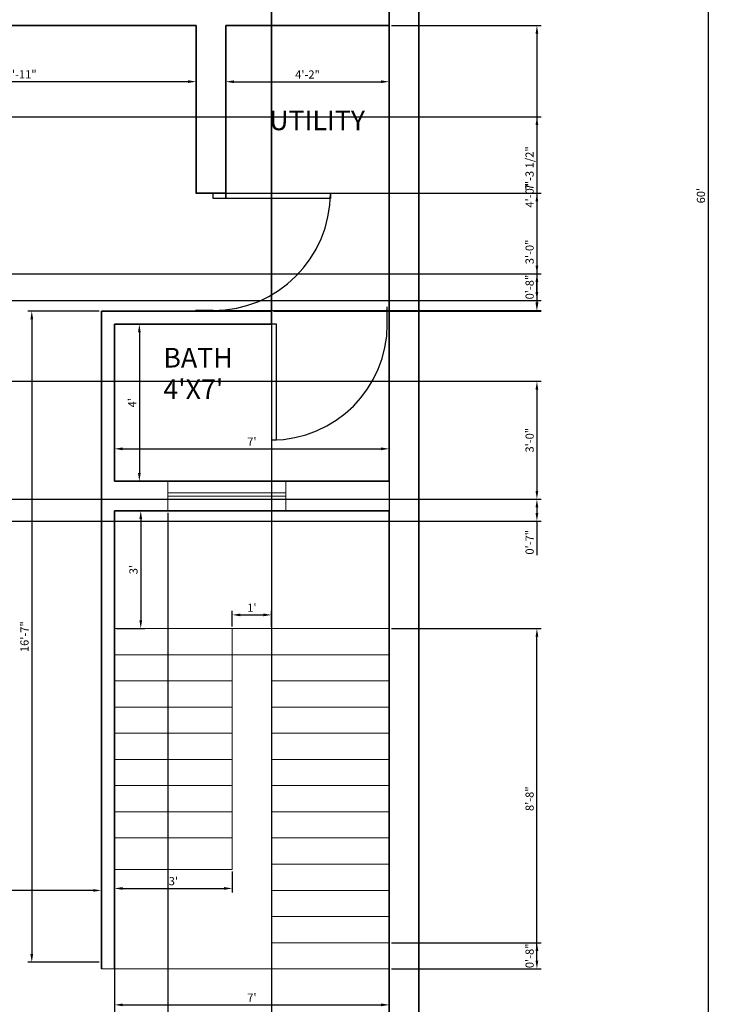
# Model space of a CAD drawing. Units: inches. Extents: x 2178 to 2667, y 1439 to 2239.
# Tile 3 of 5: x 2456 to 2667, y 1590 to 1891. Entities that reach past the tile are written whole.
import ezdxf

# ---------------------------------------------------------------- set-up
doc = ezdxf.new("R2010")
doc.units = ezdxf.units.IN
for name, color, linetype, lineweight in [('A-ANNO-DIMS', 2, 'Continuous', 18), ('A-AREA-IDEN', 7, 'Continuous', 18), ('A-DOOR', 3, 'Continuous', 25), ('A-FLOR-STRS', 7, 'Continuous', 18), ('A-GLAZ', 4, 'Continuous', 18), ('A-WALL', 7, 'Continuous', 35)]:
    doc.layers.add(name, color=color, linetype=linetype, lineweight=lineweight)
doc.styles.get("Standard").update_dxf_attribs({"font": 'arial.ttf'})
doc.dimstyles.new('Copy of ISO-25', dxfattribs={"dimtxt": 2.5, "dimasz": 2.5, "dimexe": 1.25, "dimexo": 0.625, "dimtad": 1, "dimdec": 1, "dimlunit": 4, "dimtxsty": 'Standard', "dimcen": 2.5, "dimadec": 0, "dimazin": 0, "dimtfac": 1, "dimtdec": 1, "dimtmove": 0, "dimatfit": 3, "dimfxl": 1, "dimarcsym": 0})

# ---------------------------------------------------------------- blocks, each defined once
blk = doc.blocks.new('*D14')
at = {"layer": 'A-ANNO-DIMS', "color": 0, "lineweight": -2, "transparency": 16777216}
for p, q in [((2402.53, 1888.41), (2402.53, 1870.62)), ((2509.53, 1888.41), (2509.53, 1870.62)), ((2405.03, 1871.87), (2507.03, 1871.87))]:
    blk.add_line(p, q, dxfattribs=at)
at = {"layer": 'A-ANNO-DIMS', "color": 0, "transparency": 16777216}
for points in [[(2405.03, 1872.29), (2405.03, 1871.45), (2402.53, 1871.87)], [(2507.03, 1872.29), (2507.03, 1871.45), (2509.53, 1871.87)]]:
    blk.add_solid(points, dxfattribs=at)
at = {"layer": 'Defpoints', "color": 0, "transparency": 16777216}
for p in [(2402.53, 1889.03), (2509.53, 1889.03), (2509.53, 1871.87)]:
    blk.add_point(p, dxfattribs=at)
at = {"layer": 'A-ANNO-DIMS', "color": 0, "transparency": 16777216, "insert": (2456.03, 1873.77), "char_height": 2.5, "attachment_point": 5}
blk.add_mtext('8\'-11"', dxfattribs=at)
blk = doc.blocks.new('*U22')
for p, q in [((0, 0), (0, 6)), ((40, 0), (40, 6))]:
    blk.add_line(p, q)
blk.add_lwpolyline([(0, 0), (0, -40), (1.75, -40), (1.75, 0)], close=True)
blk.add_arc((0, 0), 40, 270, 0)
blk = doc.blocks.new('*D29')
at = {"layer": 'A-ANNO-DIMS', "color": 0, "lineweight": -2, "transparency": 16777216}
for p, q in [((2402.53, 1603.39), (2402.53, 1625.96)), ((2478.03, 1624.71), (2405.03, 1624.71)), ((2480.53, 1603.39), (2480.53, 1625.96))]:
    blk.add_line(p, q, dxfattribs=at)
at = {"layer": 'A-ANNO-DIMS', "color": 0, "transparency": 16777216}
for points in [[(2405.03, 1625.13), (2405.03, 1624.3), (2402.53, 1624.71)], [(2478.03, 1625.13), (2478.03, 1624.3), (2480.53, 1624.71)]]:
    blk.add_solid(points, dxfattribs=at)
at = {"layer": 'Defpoints', "color": 0, "transparency": 16777216}
for p in [(2402.53, 1624.71), (2402.53, 1602.76), (2480.53, 1602.76)]:
    blk.add_point(p, dxfattribs=at)
at = {"layer": 'A-ANNO-DIMS', "color": 0, "transparency": 16777216, "insert": (2441.53, 1626.61), "char_height": 2.5, "attachment_point": 5}
blk.add_mtext('6\'-6"', dxfattribs=at)
blk = doc.blocks.new('*D30')
at = {"layer": 'A-ANNO-DIMS', "color": 0, "lineweight": -2, "transparency": 16777216}
for p, q in [((2479.9, 1801.74), (2458.02, 1801.74)), ((2459.27, 1799.24), (2459.27, 1605.26)), ((2479.9, 1602.76), (2458.02, 1602.76))]:
    blk.add_line(p, q, dxfattribs=at)
at = {"layer": 'A-ANNO-DIMS', "color": 0, "transparency": 16777216}
for points in [[(2458.86, 1799.24), (2459.69, 1799.24), (2459.27, 1801.74)], [(2458.86, 1605.26), (2459.69, 1605.26), (2459.27, 1602.76)]]:
    blk.add_solid(points, dxfattribs=at)
at = {"layer": 'Defpoints', "color": 0, "transparency": 16777216}
for p in [(2480.53, 1801.74), (2459.27, 1602.76), (2480.53, 1602.76)]:
    blk.add_point(p, dxfattribs=at)
at = {"layer": 'A-ANNO-DIMS', "color": 0, "transparency": 16777216, "insert": (2457.37, 1702.25), "char_height": 2.5, "attachment_point": 5, "rotation": 90}
blk.add_mtext('16\'-7"', dxfattribs=at)
blk = doc.blocks.new('*D31')
at = {"layer": 'A-ANNO-DIMS', "color": 0, "lineweight": -2, "transparency": 16777216}
for p, q in [((2484.53, 1600.12), (2484.53, 1588.5)), ((2568.53, 1600.12), (2568.53, 1588.5)), ((2487.03, 1589.75), (2566.03, 1589.75))]:
    blk.add_line(p, q, dxfattribs=at)
at = {"layer": 'A-ANNO-DIMS', "color": 0, "transparency": 16777216}
for points in [[(2487.03, 1590.17), (2487.03, 1589.33), (2484.53, 1589.75)], [(2566.03, 1590.17), (2566.03, 1589.33), (2568.53, 1589.75)]]:
    blk.add_solid(points, dxfattribs=at)
at = {"layer": 'Defpoints', "color": 0, "transparency": 16777216}
for p in [(2484.53, 1600.74), (2568.53, 1600.74), (2568.53, 1589.75)]:
    blk.add_point(p, dxfattribs=at)
at = {"layer": 'A-ANNO-DIMS', "color": 0, "transparency": 16777216, "insert": (2526.53, 1591.63), "char_height": 2.5, "attachment_point": 5}
blk.add_mtext("7'", dxfattribs=at)
blk = doc.blocks.new('*D32')
at = {"layer": 'A-ANNO-DIMS', "color": 0, "lineweight": -2, "transparency": 16777216}
for p, q in [((2485.15, 1740.74), (2493.82, 1740.74)), ((2492.57, 1738.24), (2492.57, 1707.24)), ((2485.15, 1704.74), (2493.82, 1704.74))]:
    blk.add_line(p, q, dxfattribs=at)
at = {"layer": 'A-ANNO-DIMS', "color": 0, "transparency": 16777216}
for points in [[(2492.16, 1738.24), (2492.99, 1738.24), (2492.57, 1740.74)], [(2492.16, 1707.24), (2492.99, 1707.24), (2492.57, 1704.74)]]:
    blk.add_solid(points, dxfattribs=at)
at = {"layer": 'Defpoints', "color": 0, "transparency": 16777216}
for p in [(2484.53, 1740.74), (2484.53, 1704.74), (2492.57, 1704.74)]:
    blk.add_point(p, dxfattribs=at)
at = {"layer": 'A-ANNO-DIMS', "color": 0, "transparency": 16777216, "insert": (2490.67, 1722.74), "char_height": 2.5, "attachment_point": 5, "rotation": 90}
blk.add_mtext("3'", dxfattribs=at)
blk = doc.blocks.new('*D33')
at = {"layer": 'A-ANNO-DIMS', "color": 0, "lineweight": -2, "transparency": 16777216}
for p, q in [((2485.15, 1797.74), (2493.39, 1797.74)), ((2492.14, 1795.24), (2492.14, 1752.24)), ((2485.15, 1749.74), (2493.39, 1749.74))]:
    blk.add_line(p, q, dxfattribs=at)
at = {"layer": 'A-ANNO-DIMS', "color": 0, "transparency": 16777216}
for points in [[(2491.73, 1795.24), (2492.56, 1795.24), (2492.14, 1797.74)], [(2491.73, 1752.24), (2492.56, 1752.24), (2492.14, 1749.74)]]:
    blk.add_solid(points, dxfattribs=at)
at = {"layer": 'Defpoints', "color": 0, "transparency": 16777216}
for p in [(2484.53, 1797.74), (2484.53, 1749.74), (2492.14, 1749.74)]:
    blk.add_point(p, dxfattribs=at)
at = {"layer": 'A-ANNO-DIMS', "color": 0, "transparency": 16777216, "insert": (2490.27, 1773.74), "char_height": 2.5, "attachment_point": 5, "rotation": 90}
blk.add_mtext("4'", dxfattribs=at)
blk = doc.blocks.new('*D34')
at = {"layer": 'A-ANNO-DIMS', "color": 0, "lineweight": -2, "transparency": 16777216}
for p, q in [((2484.53, 1750.37), (2484.53, 1760.9)), ((2568.53, 1750.37), (2568.53, 1760.9)), ((2487.03, 1759.65), (2566.03, 1759.65))]:
    blk.add_line(p, q, dxfattribs=at)
at = {"layer": 'A-ANNO-DIMS', "color": 0, "transparency": 16777216}
for points in [[(2487.03, 1760.07), (2487.03, 1759.23), (2484.53, 1759.65)], [(2566.03, 1760.07), (2566.03, 1759.23), (2568.53, 1759.65)]]:
    blk.add_solid(points, dxfattribs=at)
at = {"layer": 'Defpoints', "color": 0, "transparency": 16777216}
for p in [(2568.53, 1759.65), (2484.53, 1749.74), (2568.53, 1749.74)]:
    blk.add_point(p, dxfattribs=at)
at = {"layer": 'A-ANNO-DIMS', "color": 0, "transparency": 16777216, "insert": (2526.53, 1761.52), "char_height": 2.5, "attachment_point": 5}
blk.add_mtext("7'", dxfattribs=at)
blk = doc.blocks.new('*D35')
at = {"layer": 'A-ANNO-DIMS', "color": 0, "lineweight": -2, "transparency": 16777216}
for p, q in [((2518.53, 1888.41), (2518.53, 1870.58)), ((2568.53, 1888.41), (2568.53, 1870.58)), ((2521.03, 1871.83), (2566.03, 1871.83))]:
    blk.add_line(p, q, dxfattribs=at)
at = {"layer": 'A-ANNO-DIMS', "color": 0, "transparency": 16777216}
for points in [[(2521.03, 1872.25), (2521.03, 1871.42), (2518.53, 1871.83)], [(2566.03, 1872.25), (2566.03, 1871.42), (2568.53, 1871.83)]]:
    blk.add_solid(points, dxfattribs=at)
at = {"layer": 'Defpoints', "color": 0, "transparency": 16777216}
for p in [(2518.53, 1889.03), (2568.53, 1889.03), (2568.53, 1871.83)]:
    blk.add_point(p, dxfattribs=at)
at = {"layer": 'A-ANNO-DIMS', "color": 0, "transparency": 16777216, "insert": (2543.53, 1873.71), "char_height": 2.5, "attachment_point": 5}
blk.add_mtext('4\'-2"', dxfattribs=at)
blk = doc.blocks.new('*U23')
for p, q in [((-40, 0), (-40, 6)), ((0, 0), (0, 6))]:
    blk.add_line(p, q)
blk.add_lwpolyline([(0, 0), (0, -40), (-1.75, -40), (-1.75, 0)], close=True)
blk.add_arc((0, 0), 40, 180, 270)
blk = doc.blocks.new('*D38')
at = {"layer": 'A-ANNO-DIMS', "color": 0, "lineweight": -2, "transparency": 16777216}
for p, q in [((2484.53, 1630.51), (2484.53, 1624.07)), ((2520.53, 1630.51), (2520.53, 1624.07)), ((2487.03, 1625.32), (2518.03, 1625.32))]:
    blk.add_line(p, q, dxfattribs=at)
at = {"layer": 'A-ANNO-DIMS', "color": 0, "transparency": 16777216}
for points in [[(2487.03, 1625.74), (2487.03, 1624.91), (2484.53, 1625.32)], [(2518.03, 1625.74), (2518.03, 1624.91), (2520.53, 1625.32)]]:
    blk.add_solid(points, dxfattribs=at)
at = {"layer": 'Defpoints', "color": 0, "transparency": 16777216}
for p in [(2484.53, 1631.13), (2520.53, 1631.13), (2520.53, 1625.32)]:
    blk.add_point(p, dxfattribs=at)
at = {"layer": 'A-ANNO-DIMS', "color": 0, "transparency": 16777216, "insert": (2502.53, 1627.23), "char_height": 2.5, "attachment_point": 5}
blk.add_mtext("3'", dxfattribs=at)
blk = doc.blocks.new('*D39')
at = {"layer": 'A-ANNO-DIMS', "color": 0, "lineweight": -2, "transparency": 16777216}
for p, q in [((2520.53, 1705.37), (2520.53, 1710.16)), ((2532.53, 1705.37), (2532.53, 1710.16)), ((2523.03, 1708.91), (2530.03, 1708.91))]:
    blk.add_line(p, q, dxfattribs=at)
at = {"layer": 'A-ANNO-DIMS', "color": 0, "transparency": 16777216}
for points in [[(2523.03, 1709.33), (2523.03, 1708.49), (2520.53, 1708.91)], [(2530.03, 1709.33), (2530.03, 1708.49), (2532.53, 1708.91)]]:
    blk.add_solid(points, dxfattribs=at)
at = {"layer": 'Defpoints', "color": 0, "transparency": 16777216}
for p in [(2532.53, 1708.91), (2520.53, 1704.74), (2532.53, 1704.74)]:
    blk.add_point(p, dxfattribs=at)
at = {"layer": 'A-ANNO-DIMS', "color": 0, "transparency": 16777216, "insert": (2526.53, 1710.79), "char_height": 2.5, "attachment_point": 5}
blk.add_mtext("1'", dxfattribs=at)
blk = doc.blocks.new('*D41')
at = {"layer": 'A-ANNO-DIMS', "color": 0, "lineweight": -2, "transparency": 16777216}
for p, q in [((2578.15, 2197.03), (2667.22, 2197.03)), ((2665.97, 2194.53), (2665.97, 1479.53)), ((2578.15, 1477.03), (2667.22, 1477.03))]:
    blk.add_line(p, q, dxfattribs=at)
at = {"layer": 'A-ANNO-DIMS', "color": 0, "transparency": 16777216}
for points in [[(2665.56, 2194.53), (2666.39, 2194.53), (2665.97, 2197.03)], [(2665.56, 1479.53), (2666.39, 1479.53), (2665.97, 1477.03)]]:
    blk.add_solid(points, dxfattribs=at)
at = {"layer": 'Defpoints', "color": 0, "transparency": 16777216}
for p in [(2577.53, 2197.03), (2577.53, 1477.03), (2665.97, 1477.03)]:
    blk.add_point(p, dxfattribs=at)
at = {"layer": 'A-ANNO-DIMS', "color": 0, "transparency": 16777216, "insert": (2664.07, 1837.03), "char_height": 2.5, "attachment_point": 5, "rotation": 90}
blk.add_mtext("60'", dxfattribs=at)
blk = doc.blocks.new('WIN-36IN')
for p, q in [((0, 0), (0, 9)), ((36, 9), (36, 0)), ((0, 5.5), (36, 5.5)), ((0, 4.5), (36, 4.5)), ((0, 3.5), (36, 3.5)), ((36, 0), (0, 0))]:
    blk.add_line(p, q)
blk = doc.blocks.new('*D50')
at = {"layer": 'A-ANNO-DIMS', "color": 0, "lineweight": -2, "transparency": 16777216}
for p, q in [((2569.15, 1889.03), (2614.88, 1889.03)), ((2613.63, 1886.53), (2613.63, 1804.24)), ((2533.15, 1801.74), (2614.88, 1801.74))]:
    blk.add_line(p, q, dxfattribs=at)
at = {"layer": 'A-ANNO-DIMS', "color": 0, "transparency": 16777216}
for points in [[(2613.21, 1886.53), (2614.04, 1886.53), (2613.63, 1889.03)], [(2613.21, 1804.24), (2614.04, 1804.24), (2613.63, 1801.74)]]:
    blk.add_solid(points, dxfattribs=at)
at = {"layer": 'Defpoints', "color": 0, "transparency": 16777216}
for p in [(2568.53, 1889.03), (2532.53, 1801.74), (2613.63, 1801.74)]:
    blk.add_point(p, dxfattribs=at)
at = {"layer": 'A-ANNO-DIMS', "color": 0, "transparency": 16777216, "insert": (2611.71, 1845.39), "char_height": 2.5, "attachment_point": 5, "rotation": 90}
blk.add_mtext('7\'-3 1/2"', dxfattribs=at)
blk = doc.blocks.new('*D53')
at = {"layer": 'A-ANNO-DIMS', "color": 0, "lineweight": -2, "transparency": 16777216}
for p, q in [((2274.15, 1861.13), (2614.88, 1861.13)), ((2613.63, 1858.63), (2613.63, 1815.63)), ((2274.15, 1813.13), (2614.88, 1813.13))]:
    blk.add_line(p, q, dxfattribs=at)
at = {"layer": 'A-ANNO-DIMS', "color": 0, "transparency": 16777216}
for points in [[(2613.21, 1858.63), (2614.04, 1858.63), (2613.63, 1861.13)], [(2613.21, 1815.63), (2614.04, 1815.63), (2613.63, 1813.13)]]:
    blk.add_solid(points, dxfattribs=at)
at = {"layer": 'Defpoints', "color": 0, "transparency": 16777216}
for p in [(2273.53, 1861.13), (2273.53, 1813.13), (2613.63, 1813.13)]:
    blk.add_point(p, dxfattribs=at)
at = {"layer": 'A-ANNO-DIMS', "color": 0, "transparency": 16777216, "insert": (2611.72, 1837.13), "char_height": 2.5, "attachment_point": 5, "rotation": 90}
blk.add_mtext('4\'-0"', dxfattribs=at)
blk = doc.blocks.new('*D54')
at = {"layer": 'A-ANNO-DIMS', "color": 0, "lineweight": -2, "transparency": 16777216}
for p, q in [((2274.15, 1813.13), (2614.88, 1813.13)), ((2613.63, 1807.53), (2613.63, 1810.63)), ((2274.15, 1805.03), (2614.88, 1805.03))]:
    blk.add_line(p, q, dxfattribs=at)
at = {"layer": 'A-ANNO-DIMS', "color": 0, "transparency": 16777216}
for points in [[(2613.21, 1810.63), (2614.04, 1810.63), (2613.63, 1813.13)], [(2613.21, 1807.53), (2614.04, 1807.53), (2613.63, 1805.03)]]:
    blk.add_solid(points, dxfattribs=at)
at = {"layer": 'Defpoints', "color": 0, "transparency": 16777216}
for p in [(2273.53, 1813.13), (2613.63, 1813.13), (2273.53, 1805.03)]:
    blk.add_point(p, dxfattribs=at)
at = {"layer": 'A-ANNO-DIMS', "color": 0, "transparency": 16777216, "insert": (2611.72, 1809.08), "char_height": 2.5, "attachment_point": 5, "rotation": 90}
blk.add_mtext('0\'-8"', dxfattribs=at)
blk = doc.blocks.new('*D58')
at = {"layer": 'A-ANNO-DIMS', "color": 0, "lineweight": -2, "transparency": 16777216}
for p, q in [((2484.53, 1740.12), (2484.53, 1439.68)), ((2500.89, 1740.12), (2500.89, 1439.68)), ((2487.03, 1440.93), (2498.39, 1440.93))]:
    blk.add_line(p, q, dxfattribs=at)
at = {"layer": 'A-ANNO-DIMS', "color": 0, "transparency": 16777216}
for points in [[(2487.03, 1441.35), (2487.03, 1440.52), (2484.53, 1440.93)], [(2498.39, 1441.35), (2498.39, 1440.52), (2500.89, 1440.93)]]:
    blk.add_solid(points, dxfattribs=at)
at = {"layer": 'Defpoints', "color": 0, "transparency": 16777216}
for p in [(2484.53, 1740.74), (2500.89, 1740.74), (2500.89, 1440.93)]:
    blk.add_point(p, dxfattribs=at)
at = {"layer": 'A-ANNO-DIMS', "color": 0, "transparency": 16777216, "insert": (2492.71, 1442.85), "char_height": 2.5, "attachment_point": 5}
blk.add_mtext('1\'-4 1/2"', dxfattribs=at)
blk = doc.blocks.new('*D63')
at = {"layer": 'A-ANNO-DIMS', "color": 0, "lineweight": -2, "transparency": 16777216}
for p, q in [((2394.15, 1780.28), (2614.88, 1780.28)), ((2613.63, 1777.78), (2613.63, 1746.78)), ((2394.15, 1744.28), (2614.88, 1744.28))]:
    blk.add_line(p, q, dxfattribs=at)
at = {"layer": 'A-ANNO-DIMS', "color": 0, "transparency": 16777216}
for points in [[(2613.21, 1777.78), (2614.04, 1777.78), (2613.63, 1780.28)], [(2613.21, 1746.78), (2614.04, 1746.78), (2613.63, 1744.28)]]:
    blk.add_solid(points, dxfattribs=at)
at = {"layer": 'Defpoints', "color": 0, "transparency": 16777216}
for p in [(2393.53, 1780.28), (2393.53, 1744.28), (2613.63, 1744.28)]:
    blk.add_point(p, dxfattribs=at)
at = {"layer": 'A-ANNO-DIMS', "color": 0, "transparency": 16777216, "insert": (2611.72, 1762.28), "char_height": 2.5, "attachment_point": 5, "rotation": 90}
blk.add_mtext('3\'-0"', dxfattribs=at)
blk = doc.blocks.new('*D64')
at = {"layer": 'A-ANNO-DIMS', "color": 0, "lineweight": -2, "transparency": 16777216}
for p, q in [((2394.15, 1744.28), (2614.88, 1744.28)), ((2613.63, 1741.78), (2613.63, 1740.03)), ((2394.15, 1737.53), (2614.88, 1737.53)), ((2613.63, 1737.53), (2613.63, 1727.14))]:
    blk.add_line(p, q, dxfattribs=at)
at = {"layer": 'A-ANNO-DIMS', "color": 0, "transparency": 16777216}
for points in [[(2613.21, 1741.78), (2614.04, 1741.78), (2613.63, 1744.28)], [(2613.21, 1740.03), (2614.04, 1740.03), (2613.63, 1737.53)]]:
    blk.add_solid(points, dxfattribs=at)
at = {"layer": 'Defpoints', "color": 0, "transparency": 16777216}
for p in [(2393.53, 1744.28), (2393.53, 1737.53), (2613.63, 1737.53)]:
    blk.add_point(p, dxfattribs=at)
at = {"layer": 'A-ANNO-DIMS', "color": 0, "transparency": 16777216, "insert": (2611.72, 1731.09), "char_height": 2.5, "attachment_point": 5, "rotation": 90}
blk.add_mtext('0\'-7"', dxfattribs=at)
blk = doc.blocks.new('*D65')
at = {"layer": 'A-ANNO-DIMS', "color": 0, "lineweight": -2, "transparency": 16777216}
for p, q in [((2569.15, 1704.74), (2614.88, 1704.74)), ((2613.63, 1603.24), (2613.63, 1702.24)), ((2569.15, 1600.74), (2614.88, 1600.74))]:
    blk.add_line(p, q, dxfattribs=at)
at = {"layer": 'A-ANNO-DIMS', "color": 0, "transparency": 16777216}
for points in [[(2613.21, 1702.24), (2614.04, 1702.24), (2613.63, 1704.74)], [(2613.21, 1603.24), (2614.04, 1603.24), (2613.63, 1600.74)]]:
    blk.add_solid(points, dxfattribs=at)
at = {"layer": 'Defpoints', "color": 0, "transparency": 16777216}
for p in [(2568.53, 1704.74), (2613.63, 1704.74), (2568.53, 1600.74)]:
    blk.add_point(p, dxfattribs=at)
at = {"layer": 'A-ANNO-DIMS', "color": 0, "transparency": 16777216, "insert": (2611.72, 1652.74), "char_height": 2.5, "attachment_point": 5, "rotation": 90}
blk.add_mtext('8\'-8"', dxfattribs=at)
blk = doc.blocks.new('*D66')
at = {"layer": 'A-ANNO-DIMS', "color": 0, "lineweight": -2, "transparency": 16777216}
for p, q in [((2569.15, 1608.74), (2614.88, 1608.74)), ((2613.63, 1603.24), (2613.63, 1606.24)), ((2569.15, 1600.74), (2614.88, 1600.74))]:
    blk.add_line(p, q, dxfattribs=at)
at = {"layer": 'A-ANNO-DIMS', "color": 0, "transparency": 16777216}
for points in [[(2613.21, 1606.24), (2614.04, 1606.24), (2613.63, 1608.74)], [(2613.21, 1603.24), (2614.04, 1603.24), (2613.63, 1600.74)]]:
    blk.add_solid(points, dxfattribs=at)
at = {"layer": 'Defpoints', "color": 0, "transparency": 16777216}
for p in [(2568.53, 1608.74), (2613.63, 1608.74), (2568.53, 1600.74)]:
    blk.add_point(p, dxfattribs=at)
at = {"layer": 'A-ANNO-DIMS', "color": 0, "transparency": 16777216, "insert": (2611.72, 1604.74), "char_height": 2.5, "attachment_point": 5, "rotation": 90}
blk.add_mtext('0\'-8"', dxfattribs=at)
blk = doc.blocks.new('*D70')
at = {"layer": 'A-ANNO-DIMS', "color": 0, "lineweight": -2, "transparency": 16777216}
for p, q in [((2532.53, 1798.37), (2532.53, 2234.38)), ((2535.03, 2233.13), (2566.03, 2233.13)), ((2568.53, 1798.37), (2568.53, 2234.38))]:
    blk.add_line(p, q, dxfattribs=at)
at = {"layer": 'A-ANNO-DIMS', "color": 0, "transparency": 16777216}
for points in [[(2535.03, 2233.55), (2535.03, 2232.72), (2532.53, 2233.13)], [(2566.03, 2233.55), (2566.03, 2232.72), (2568.53, 2233.13)]]:
    blk.add_solid(points, dxfattribs=at)
at = {"layer": 'Defpoints', "color": 0, "transparency": 16777216}
for p in [(2568.53, 2233.13), (2532.53, 1797.74), (2568.53, 1797.74)]:
    blk.add_point(p, dxfattribs=at)
at = {"layer": 'A-ANNO-DIMS', "color": 0, "transparency": 16777216, "insert": (2550.53, 2235.04), "char_height": 2.5, "attachment_point": 5}
blk.add_mtext('3\'-0"', dxfattribs=at)
blk = doc.blocks.new('*D72')
at = {"layer": 'A-ANNO-DIMS', "color": 0, "lineweight": -2, "transparency": 16777216}
for p, q in [((2519.15, 1837.74), (2614.88, 1837.74)), ((2613.63, 1835.24), (2613.63, 1804.4)), ((2515.28, 1801.9), (2614.88, 1801.9))]:
    blk.add_line(p, q, dxfattribs=at)
at = {"layer": 'A-ANNO-DIMS', "color": 0, "transparency": 16777216}
for points in [[(2613.21, 1835.24), (2614.04, 1835.24), (2613.63, 1837.74)], [(2613.21, 1804.4), (2614.04, 1804.4), (2613.63, 1801.9)]]:
    blk.add_solid(points, dxfattribs=at)
at = {"layer": 'Defpoints', "color": 0, "transparency": 16777216}
for p in [(2518.53, 1837.74), (2514.66, 1801.9), (2613.63, 1801.9)]:
    blk.add_point(p, dxfattribs=at)
at = {"layer": 'A-ANNO-DIMS', "color": 0, "transparency": 16777216, "insert": (2611.72, 1819.82), "char_height": 2.5, "attachment_point": 5, "rotation": 90}
blk.add_mtext('3\'-0"', dxfattribs=at)
blk = doc.blocks.new('*D73')
at = {"layer": 'A-ANNO-DIMS', "color": 0, "lineweight": -2, "transparency": 16777216}
for p, q in [((2568.53, 2187.41), (2568.53, 1439.68)), ((2532.53, 2128.41), (2532.53, 1439.68)), ((2535.03, 1440.93), (2566.03, 1440.93))]:
    blk.add_line(p, q, dxfattribs=at)
at = {"layer": 'A-ANNO-DIMS', "color": 0, "transparency": 16777216}
for points in [[(2535.03, 1441.35), (2535.03, 1440.52), (2532.53, 1440.93)], [(2566.03, 1441.35), (2566.03, 1440.52), (2568.53, 1440.93)]]:
    blk.add_solid(points, dxfattribs=at)
at = {"layer": 'Defpoints', "color": 0, "transparency": 16777216}
for p in [(2568.53, 2188.03), (2532.53, 2129.03), (2568.53, 1440.93)]:
    blk.add_point(p, dxfattribs=at)
at = {"layer": 'A-ANNO-DIMS', "color": 0, "transparency": 16777216, "insert": (2550.53, 1442.84), "char_height": 2.5, "attachment_point": 5}
blk.add_mtext('3\'-0"', dxfattribs=at)

msp = doc.modelspace()

# ---------------------------------------------------------------- linework, layer by layer
at = {"layer": 'A-FLOR-STRS'}
for p, q in [((2484.53, 1740.74), (2484.53, 1704.74)), ((2484.53, 1704.74), (2568.53, 1704.74)), ((2484.53, 1704.74), (2520.53, 1704.74)), ((2484.53, 1704.74), (2484.53, 1696.74)), ((2520.53, 1704.74), (2520.53, 1631.13)), ((2568.53, 1704.74), (2532.53, 1704.74)), ((2532.53, 1704.74), (2532.53, 1600.74)), ((2484.53, 1696.74), (2520.53, 1696.74)), ((2520.53, 1696.74), (2520.53, 1688.74)), ((2520.53, 1696.74), (2532.53, 1696.74)), ((2532.53, 1696.74), (2568.53, 1696.74)), ((2568.53, 1696.74), (2568.53, 1688.74)), ((2520.53, 1688.74), (2484.53, 1688.74)), ((2484.53, 1688.74), (2484.53, 1680.74)), ((2568.53, 1688.74), (2532.53, 1688.74)), ((2532.53, 1688.74), (2532.53, 1680.74)), ((2484.53, 1680.74), (2520.53, 1680.74)), ((2520.53, 1680.74), (2520.53, 1672.74)), ((2532.53, 1680.74), (2568.53, 1680.74)), ((2568.53, 1680.74), (2568.53, 1672.74)), ((2520.53, 1672.74), (2484.53, 1672.74)), ((2484.53, 1672.74), (2484.53, 1664.74)), ((2568.53, 1672.74), (2532.53, 1672.74)), ((2532.53, 1672.74), (2532.53, 1664.74)), ((2484.53, 1664.74), (2520.53, 1664.74)), ((2520.53, 1664.74), (2520.53, 1656.74)), ((2532.53, 1664.74), (2568.53, 1664.74)), ((2568.53, 1664.74), (2568.53, 1656.74)), ((2520.53, 1656.74), (2484.53, 1656.74)), ((2484.53, 1656.74), (2484.53, 1648.74)), ((2568.53, 1656.74), (2532.53, 1656.74)), ((2532.53, 1656.74), (2532.53, 1648.74)), ((2484.53, 1648.74), (2520.53, 1648.74)), ((2520.53, 1648.74), (2520.53, 1640.74)), ((2532.53, 1648.74), (2568.53, 1648.74)), ((2568.53, 1648.74), (2568.53, 1640.74)), ((2520.53, 1640.74), (2484.53, 1640.74)), ((2568.53, 1640.74), (2532.53, 1640.74)), ((2532.53, 1640.74), (2532.53, 1632.74)), ((2520.53, 1631.13), (2484.53, 1631.13)), ((2532.53, 1632.74), (2568.53, 1632.74)), ((2568.53, 1632.74), (2568.53, 1624.74)), ((2568.53, 1624.74), (2532.53, 1624.74)), ((2532.53, 1624.74), (2532.53, 1616.74)), ((2532.53, 1616.74), (2568.53, 1616.74)), ((2568.53, 1616.74), (2568.53, 1608.74)), ((2568.53, 1608.74), (2532.53, 1608.74)), ((2532.53, 1608.74), (2532.53, 1600.74)), ((2532.53, 1600.74), (2480.53, 1600.74)), ((2532.53, 1600.74), (2568.53, 1600.74))]:
    msp.add_line(p, q, dxfattribs=at)
at = {"layer": 'A-WALL'}
for p, q in [((2577.53, 2197.03), (2577.53, 1477.03)), ((2568.53, 2188.03), (2568.53, 1749.74)), ((2568.53, 1889.03), (2568.53, 1898.03)), ((2374.53, 1889.03), (2509.53, 1889.03)), ((2509.53, 1889.03), (2402.53, 1889.03)), ((2509.53, 1837.74), (2509.53, 1889.03)), ((2568.53, 1889.03), (2518.53, 1889.03)), ((2518.53, 1889.03), (2518.53, 1837.74)), ((2518.53, 1889.03), (2568.53, 1889.03)), ((2518.53, 1837.74), (2509.53, 1837.74)), ((2518.53, 1837.74), (2518.53, 1836.18)), ((2484.53, 1801.74), (2480.53, 1801.74)), ((2480.53, 1801.74), (2480.53, 1749.74)), ((2509.53, 1801.74), (2484.53, 1801.74)), ((2532.53, 1801.74), (2509.53, 1801.74)), ((2518.53, 1802.1), (2518.53, 1801.74)), ((2518.53, 1801.74), (2532.53, 1801.74)), ((2532.53, 1797.74), (2532.53, 1801.74)), ((2532.53, 1797.74), (2484.53, 1797.74)), ((2484.53, 1797.74), (2484.53, 1749.74)), ((2509.53, 1797.74), (2532.53, 1797.74)), ((2568.53, 1797.74), (2568.53, 1749.74)), ((2480.53, 1749.74), (2480.53, 1740.74)), ((2484.53, 1749.74), (2509.53, 1749.74)), ((2484.53, 1749.74), (2500.89, 1749.74)), ((2568.53, 1749.74), (2509.53, 1749.74)), ((2480.53, 1740.74), (2480.53, 1600.74)), ((2484.53, 1740.74), (2509.53, 1740.74)), ((2484.53, 1600.74), (2484.53, 1740.74)), ((2509.53, 1740.74), (2568.53, 1740.74)), ((2568.53, 1740.74), (2568.53, 1486.03))]:
    msp.add_line(p, q, dxfattribs=at)

# ---------------------------------------------------------------- block references
at = {"layer": 'A-DOOR', "xscale": 0.896210211266654, "yscale": 0.896210211266654, "zscale": 0.896210211266654, "rotation": 90}
msp.add_blockref('*U23', (2514.66, 1837.74), dxfattribs=at)
at = {"layer": 'A-DOOR', "xscale": 0.8844272464074808, "yscale": 0.8844272464074808, "zscale": 0.8844272464074808}
msp.add_blockref('*U22', (2532.53, 1797.74), dxfattribs=at)
at = {"layer": 'A-GLAZ'}
msp.add_blockref('WIN-36IN', (2500.89, 1740.74), dxfattribs=at)

# ---------------------------------------------------------------- texts
at = {"layer": 'A-AREA-IDEN'}
for s, p in [('UTILITY', (2531.82, 1857.02)), ('BATH', (2499.47, 1784.5)), ("4'X7'", (2499.47, 1774.86))]:
    msp.add_text(s, height=6, dxfattribs=at).set_placement(p)

# ---------------------------------------------------------------- dimensions: what is measured, and where the dimension line sits
at = {"layer": 'A-ANNO-DIMS'}
for base, p1, p2, override, picture, middle in [((2568.53, 2233.13), (2532.53, 1797.74), (2568.53, 1797.74), {"dimdec": 1, "dimlfac": 1, "dimrnd": 0, "dimzin": 1, "dimdsep": 46, "dimlunit": 4, "dimfrac": 2}, '*D70', (2550.53, 2235.04)), ((2568.53, 1440.93), (2532.53, 2129.03), (2568.53, 2188.03), {"dimdec": 1, "dimlfac": 1, "dimrnd": 0, "dimzin": 1, "dimdsep": 46, "dimlunit": 4, "dimfrac": 2}, '*D73', (2550.53, 1442.84)), ((2509.53, 1871.87), (2402.53, 1889.03), (2509.53, 1889.03), {"dimclrd": 0, "dimclre": 0, "dimclrt": 0}, '*D14', (2456.03, 1873.77)), ((2568.53, 1871.83), (2518.53, 1889.03), (2568.53, 1889.03), {"dimclrd": 0, "dimclre": 0, "dimclrt": 0}, '*D35', (2543.53, 1873.71)), ((2568.53, 1759.65), (2484.53, 1749.74), (2568.53, 1749.74), {"dimclrd": 0, "dimclre": 0, "dimclrt": 0}, '*D34', (2526.53, 1761.52)), ((2500.89, 1440.93), (2484.53, 1740.74), (2500.89, 1740.74), {"dimdec": 1, "dimlfac": 1, "dimrnd": 0, "dimzin": 1, "dimdsep": 46, "dimlunit": 4, "dimfrac": 2}, '*D58', (2492.71, 1442.85)), ((2532.53, 1708.91), (2520.53, 1704.74), (2532.53, 1704.74), {"dimclrd": 0, "dimclre": 0, "dimclrt": 0}, '*D39', (2526.53, 1710.79)), ((2520.53, 1625.32), (2484.53, 1631.13), (2520.53, 1631.13), {"dimclrd": 0, "dimclre": 0, "dimclrt": 0}, '*D38', (2502.53, 1627.23)), ((2402.53, 1624.71), (2480.53, 1602.76), (2402.53, 1602.76), {"dimclrd": 0, "dimclre": 0, "dimclrt": 0}, '*D29', (2441.53, 1626.61)), ((2568.53, 1589.75), (2484.53, 1600.74), (2568.53, 1600.74), {"dimclrd": 0, "dimclre": 0, "dimclrt": 0}, '*D31', (2526.53, 1591.63))]:
    dim = msp.add_linear_dim(base=base, p1=p1, p2=p2, dimstyle='Copy of ISO-25', override=override, dxfattribs=at)
    dim.commit()
    dim.dimension.update_dxf_attribs({"geometry": picture, "text_midpoint": middle})
for base, p1, p2, override, picture, middle in [((2665.97, 1477.03), (2577.53, 2197.03), (2577.53, 1477.03), {"dimclrd": 0, "dimclre": 0, "dimclrt": 0}, '*D41', (2664.07, 1837.03)), ((2613.63, 1801.74), (2568.53, 1889.03), (2532.53, 1801.74), {"dimdec": 1, "dimlfac": 1, "dimrnd": 0, "dimzin": 1, "dimdsep": 46, "dimlunit": 4, "dimfrac": 2}, '*D50', (2611.71, 1845.39)), ((2613.63, 1813.13), (2273.53, 1861.13), (2273.53, 1813.13), {"dimdec": 1, "dimlfac": 1, "dimrnd": 0, "dimzin": 1, "dimdsep": 46, "dimlunit": 4, "dimfrac": 2}, '*D53', (2611.72, 1837.13)), ((2613.63, 1801.9), (2518.53, 1837.74), (2514.66, 1801.9), {"dimdec": 1, "dimlfac": 1, "dimrnd": 0, "dimzin": 1, "dimdsep": 46, "dimlunit": 4, "dimfrac": 2}, '*D72', (2611.72, 1819.82)), ((2613.63, 1813.13), (2273.53, 1805.03), (2273.53, 1813.13), {"dimdec": 1, "dimlfac": 1, "dimrnd": 0, "dimzin": 1, "dimdsep": 46, "dimlunit": 4, "dimfrac": 2}, '*D54', (2611.72, 1809.08)), ((2459.27, 1602.76), (2480.53, 1801.74), (2480.53, 1602.76), {"dimclrd": 0, "dimclre": 0, "dimclrt": 0}, '*D30', (2457.37, 1702.25)), ((2492.14, 1749.74), (2484.53, 1797.74), (2484.53, 1749.74), {"dimclrd": 0, "dimclre": 0, "dimclrt": 0}, '*D33', (2490.27, 1773.74)), ((2613.63, 1744.28), (2393.53, 1780.28), (2393.53, 1744.28), {"dimdec": 1, "dimlfac": 1, "dimrnd": 0, "dimzin": 1, "dimdsep": 46, "dimlunit": 4, "dimfrac": 2}, '*D63', (2611.72, 1762.28)), ((2613.625586, 1737.534601), (2393.525586, 1744.284601), (2393.525586, 1737.534601), {"dimdec": 1, "dimlfac": 1, "dimrnd": 0, "dimzin": 1, "dimdsep": 46, "dimlunit": 4, "dimfrac": 2}, '*D64', (2611.72415353, 1731.08678381)), ((2492.57, 1704.74), (2484.53, 1740.74), (2484.53, 1704.74), {"dimclrd": 0, "dimclre": 0, "dimclrt": 0}, '*D32', (2490.67, 1722.74)), ((2613.63, 1704.74), (2568.53, 1600.74), (2568.53, 1704.74), {"dimdec": 1, "dimlfac": 1, "dimrnd": 0, "dimzin": 1, "dimdsep": 46, "dimlunit": 4, "dimfrac": 2}, '*D65', (2611.72, 1652.74)), ((2613.63, 1608.74), (2568.53, 1600.74), (2568.53, 1608.74), {"dimdec": 1, "dimlfac": 1, "dimrnd": 0, "dimzin": 1, "dimdsep": 46, "dimlunit": 4, "dimfrac": 2}, '*D66', (2611.72, 1604.74))]:
    dim = msp.add_linear_dim(base=base, p1=p1, p2=p2, angle=90, dimstyle='Copy of ISO-25', override=override, dxfattribs=at)
    dim.commit()
    dim.dimension.update_dxf_attribs({"geometry": picture, "text_midpoint": middle})

doc.saveas('drawing.dxf')
